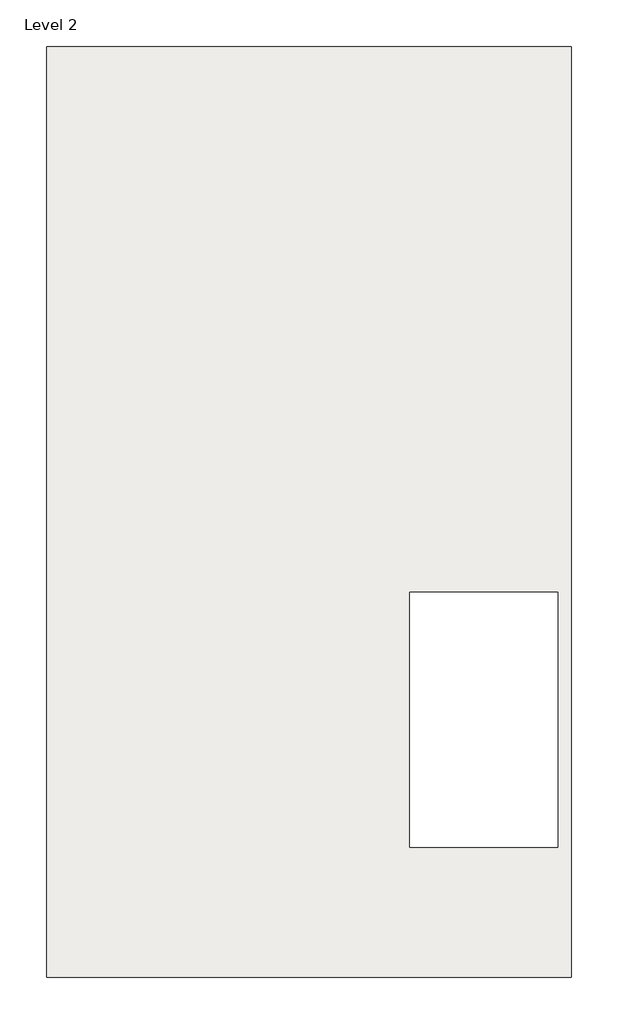
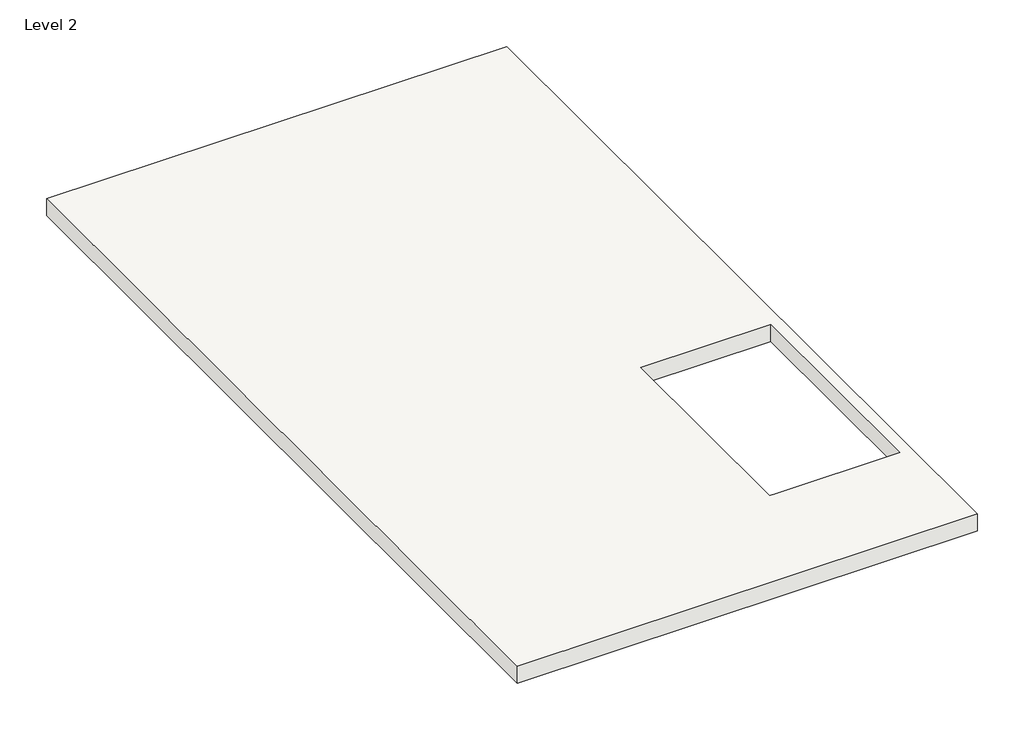
# One storey: 1 roof.
"""IFC4 building model written with IfcOpenShell, lengths in millimetres."""

from ifc_helpers import new_model, si_unit, frame, origin, place, context, project, spatial, polyline, outline, extrude, element, save

model = new_model("IFC4")

# Units and contexts
model_context = context("Model", 3, world=origin())
ifc_project = project(units=[si_unit("LENGTHUNIT", "METRE", prefix="MILLI")], contexts=[model_context])

# Site, building, storey
site = spatial("IfcSite", under=ifc_project)
building = spatial("IfcBuilding", under=site)
storey = spatial("IfcBuildingStorey", under=building, Name="Level 2", Elevation=3048.0)

# Roof
placement = place(None, origin())
element("IfcRoof", 1, ObjectType="Generic - 12\"", at=placement, inside=storey, context=model_context, shape_type="SweptSolid", body=[
    extrude(outline(polyline([(-14337.3118598, 13484.1368529), (-6488.7118598, 13484.1368529), (-6488.7118598, -435.0631471), (-14337.3118598, -435.0631471), (-14337.3118598, 13484.1368529)]), holes=[polyline([(-6691.9118598, 1511.9710899), (-6691.9118598, 5321.9710899), (-8908.3116993, 5321.9710899), (-8908.3116993, 1511.9710899), (-8825.5118598, 1511.9710899), (-6691.9118598, 1511.9710899)])]), frame((0.0, 0.0, 3048.0), z_axis=(0.0, 0.0, 1.0), x_axis=(1.0, 0.0, 0.0)), (0.0, 0.0, 1.0), 304.8),
])

save(model, "model.ifc")

# Revit data of these elements
# Type "Generic - 12\""
#   Assembly Code = "B1020"
#   Layers, outside or top first: 1' - 0" "Brick, Soldier Course" (function 1)
# Element 1 (IfcRoof, "Generic - 12\"")
#   built-in parameter 1001705 = 11 (stored number, unit not read)
#   built-in parameter 1001710 = 33615
#   Phase Created = New Construction
#   Materials on its faces: "Brick, Soldier Course"
# Materials
#   "Brick, Soldier Course": class "Masonry", colour RGB 170 98 104, transparency 0, Description = "Common brick soldier coursed", Cost = 0
